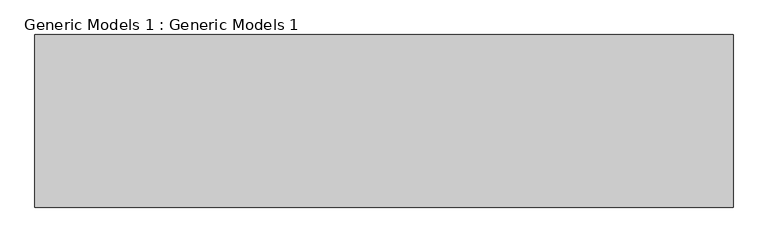
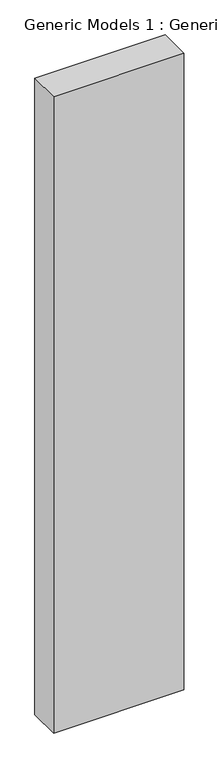
"""IFC4 building model written with IfcOpenShell, lengths in millimetres: proxy geometry, Generic Models 1 : Generic Models 1."""

from ifc_helpers import new_model, si_unit, origin, origin_with_axes, place, context, project, spatial, polyline, outline, extrude, source, transform, mapped, element, save


def generic_models_1_generic_models_1_d491554d(model_context):
    return source(origin(), model_context, "Body", "SweptSolid", [
        extrude(outline(polyline([(-1362.8128458, 1851.619734), (-1362.8128458, 1460.0626253), (-2943.862839, 1460.0626253), (-2943.862839, 1851.619734), (-1362.8128458, 1851.619734)])), origin_with_axes(), (0.0, 0.0, 1.0), 8163.0655737),
    ])


if __name__ == "__main__":
    model = new_model("IFC4")
    model_context = context("Model", 3, world=origin())
    ifc_project = project(units=[si_unit("LENGTHUNIT", "METRE", prefix="MILLI")], contexts=[model_context])
    site = spatial("IfcSite", under=ifc_project)
    building = spatial("IfcBuilding", under=site)
    placement = place(None, origin())
    generic_models_1_generic_models_1_shape = generic_models_1_generic_models_1_d491554d(model_context)
    element("IfcBuildingElementProxy", 1, Name="Generic Models 1 : Generic Models 1", ObjectType="Generic Models 1 : Generic Models 1", at=placement, inside=building, context=model_context, shape_type="MappedRepresentation", body=[
        mapped(generic_models_1_generic_models_1_shape, transform((0.0, 0.0, 0.0), x_axis=(1.0, 0.0, 0.0), y_axis=(0.0, 1.0, 0.0), z_axis=(0.0, 0.0, 1.0))),
    ])
    save(model, "model.ifc")
